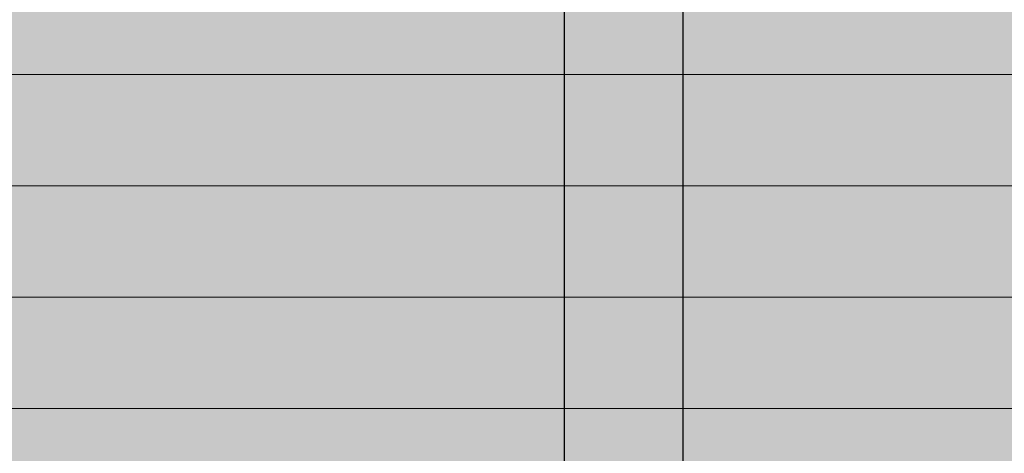
# Model space of a CAD drawing. Units: inches. Extents: x 1704 to 6393, y -157 to 1172.
# Tile 98 of 122: x 2561 to 2627, y 972 to 1001. Entities that reach past the tile are written whole.
import ezdxf

# ---------------------------------------------------------------- set-up
doc = ezdxf.new("R2010")
doc.units = ezdxf.units.IN
doc.header["$MEASUREMENT"] = 0
doc.layers.add('A-ANNO-DIMS', color=7, linetype='Continuous', lineweight=13)
doc.layers.add('L-DECK-PLNK-PATT', color=250, linetype='Continuous', lineweight=13)
doc.layers.add('L-DECK-PATT', color=35, linetype='Continuous', lineweight=13, true_color=0xa6725b)
doc.styles.get("Standard").update_dxf_attribs({"font": 'arial.ttf'})
doc.dimstyles.get("Standard").update_dxf_attribs({"dimtxt": 6, "dimasz": 2, "dimexe": 0.18, "dimexo": 0.0625, "dimgap": 0.09, "dimtad": 0, "dimtih": 1, "dimtoh": 1, "dimdec": 1, "dimzin": 0, "dimdsep": 46, "dimlunit": 3, "dimtxsty": 'Standard', "dimblk": 'ARCHTICK', "dimcen": 0.09, "dimadec": 0, "dimazin": 0, "dimtfac": 1, "dimtdec": 1, "dimtofl": 0, "dimtmove": 0, "dimatfit": 3, "dimfxl": 1, "dimtolj": 1, "dimtzin": 0, "dimarcsym": 0})

# ---------------------------------------------------------------- blocks, each defined once
blk = doc.blocks.new('_ArchTick')
at = {"color": 0, "linetype": 'ByBlock', "const_width": 0.15}
blk.add_lwpolyline([(-0.5, -0.5), (0.5, 0.5)], dxfattribs=at)
blk = doc.blocks.new('*D92')
at = {"layer": 'A-ANNO-DIMS', "color": 0, "lineweight": -2, "transparency": 16777216}
for p, q in [((2073.349, 895.275), (2073.349, 1105.287)), ((2605.349, 895.275), (2605.349, 1105.287)), ((2073.349, 1105.107), (2332.661, 1105.107)), ((2605.349, 1105.107), (2346.036, 1105.107))]:
    blk.add_line(p, q, dxfattribs=at)
at = {"layer": 'Defpoints', "color": 0, "lineweight": -3, "transparency": 16777216}
for p in [(2605.349, 1105.107), (2073.349, 895.213), (2605.349, 895.213)]:
    blk.add_point(p, dxfattribs=at)
at = {"layer": 'A-ANNO-DIMS', "color": 0, "lineweight": -2, "transparency": 16777216, "xscale": 2, "yscale": 2, "zscale": 2, "rotation": 180}
blk.add_blockref('_ArchTick', (2073.349, 1105.107), dxfattribs=at)
at = {"layer": 'A-ANNO-DIMS', "color": 0, "lineweight": -2, "transparency": 16777216, "xscale": 2, "yscale": 2, "zscale": 2}
blk.add_blockref('_ArchTick', (2605.349, 1105.107), dxfattribs=at)
at = {"layer": 'A-ANNO-DIMS', "color": 0, "transparency": 16777216, "insert": (2339.349, 1105.107), "char_height": 6, "attachment_point": 5}
blk.add_mtext('\\A1;532', dxfattribs=at)
blk = doc.blocks.new('*D95')
at = {"layer": 'A-ANNO-DIMS', "color": 0, "lineweight": -2, "transparency": 16777216}
for p, q in [((2605.349, 895.275), (2605.349, 1105.287)), ((2723.349, 895.275), (2723.349, 1105.287)), ((2605.349, 1105.107), (2657.907, 1105.107)), ((2723.349, 1105.107), (2670.791, 1105.107))]:
    blk.add_line(p, q, dxfattribs=at)
at = {"layer": 'Defpoints', "color": 0, "lineweight": -3, "transparency": 16777216}
for p in [(2723.349, 1105.107), (2605.349, 895.213), (2723.349, 895.213)]:
    blk.add_point(p, dxfattribs=at)
at = {"layer": 'A-ANNO-DIMS', "color": 0, "lineweight": -2, "transparency": 16777216, "xscale": 2, "yscale": 2, "zscale": 2, "rotation": 180}
blk.add_blockref('_ArchTick', (2605.349, 1105.107), dxfattribs=at)
at = {"layer": 'A-ANNO-DIMS', "color": 0, "lineweight": -2, "transparency": 16777216, "xscale": 2, "yscale": 2, "zscale": 2}
blk.add_blockref('_ArchTick', (2723.349, 1105.107), dxfattribs=at)
at = {"layer": 'A-ANNO-DIMS', "color": 0, "transparency": 16777216, "insert": (2664.349, 1105.107), "char_height": 6, "attachment_point": 5}
blk.add_mtext('\\A1;118', dxfattribs=at)
blk = doc.blocks.new('*D103')
at = {"layer": 'A-ANNO-DIMS', "color": 0, "lineweight": -2, "transparency": 16777216}
for p, q in [((2551.349, 711.275), (2551.349, 1105.287)), ((2597.349, 711.275), (2597.349, 1105.287)), ((2551.349, 1105.107), (2569.842, 1105.107)), ((2597.349, 1105.107), (2578.855, 1105.107))]:
    blk.add_line(p, q, dxfattribs=at)
at = {"layer": 'Defpoints', "color": 0, "lineweight": -3, "transparency": 16777216}
for p in [(2597.349, 1105.107), (2551.349, 711.213), (2597.349, 711.213)]:
    blk.add_point(p, dxfattribs=at)
at = {"layer": 'A-ANNO-DIMS', "color": 0, "lineweight": -2, "transparency": 16777216, "xscale": 2, "yscale": 2, "zscale": 2, "rotation": 180}
blk.add_blockref('_ArchTick', (2551.349, 1105.107), dxfattribs=at)
at = {"layer": 'A-ANNO-DIMS', "color": 0, "lineweight": -2, "transparency": 16777216, "xscale": 2, "yscale": 2, "zscale": 2}
blk.add_blockref('_ArchTick', (2597.349, 1105.107), dxfattribs=at)
at = {"layer": 'A-ANNO-DIMS', "color": 0, "transparency": 16777216, "insert": (2574.349, 1105.107), "char_height": 6, "attachment_point": 5}
blk.add_mtext('\\A1;46', dxfattribs=at)

msp = doc.modelspace()

# ---------------------------------------------------------------- hatches: boundary and pattern name
at = {"layer": 'L-DECK-PATT', "transparency": 33554544}
h = msp.add_hatch(color=256, dxfattribs=at)
h.dxf.hatch_style = 1
h.paths.add_polyline_path([(2329.589, 1033.213), (2065.589, 1033.213), (2065.589, 895.213), (2167.349, 895.213), (2263.349, 895.213), (2263.349, 903.213), (2273.349, 903.213), (2273.349, 895.213), (2329.589, 895.213)])
h.paths.add_polyline_path([(2664.349, 1033.213), (2333.589, 1033.213), (2333.589, 895.213), (2465.349, 895.213), (2469.181, 895.213), (2470.482, 895.213), (2508.215, 895.213), (2509.516, 895.213), (2513.349, 895.213), (2533.349, 895.213), (2581.349, 895.213), (2605.349, 895.213), (2664.349, 895.213)])
h.paths.add_polyline_path([(2333.589, 1033.213), (2329.589, 1033.213), (2329.589, 895.213), (2333.589, 895.213)])
at = {"layer": 'L-DECK-PLNK-PATT'}
h = msp.add_hatch(dxfattribs=at)
h.set_pattern_fill('LINE', color=256, scale=60)
h.paths.add_polyline_path([(2329.589, 1033.213), (2065.589, 1033.213), (2065.589, 895.213), (2167.349, 895.213), (2263.349, 895.213), (2263.349, 903.213), (2273.349, 903.213), (2273.349, 895.213), (2329.589, 895.213)])
h.paths.add_polyline_path([(2664.349, 1033.213), (2333.589, 1033.213), (2333.589, 895.213), (2465.349, 895.213), (2469.181, 895.213), (2470.482, 895.213), (2508.215, 895.213), (2509.516, 895.213), (2513.349, 895.213), (2533.349, 895.213), (2581.349, 895.213), (2605.349, 895.213), (2664.349, 895.213)])
h.paths.add_polyline_path([(2333.589, 1033.213), (2329.589, 1033.213), (2329.589, 895.213), (2333.589, 895.213)])

# ---------------------------------------------------------------- dimensions: what is measured, and where the dimension line sits
at = {"layer": 'A-ANNO-DIMS'}
for base, p1, p2, picture, middle in [((2605.349, 1105.107), (2073.349, 895.213), (2605.349, 895.213), '*D92', (2339.349, 1105.107)), ((2597.349, 1105.107), (2551.349, 711.213), (2597.349, 711.213), '*D103', (2574.349, 1105.107)), ((2723.349, 1105.107), (2605.349, 895.213), (2723.349, 895.213), '*D95', (2664.349, 1105.107))]:
    dim = msp.add_linear_dim(base=base, p1=p1, p2=p2, dimstyle='Standard', override={"dimdec": 0, "dimlfac": 1, "dimrnd": 0, "dimzin": 0, "dimdsep": 46, "dimlunit": 2}, dxfattribs=at)
    dim.commit()
    dim.dimension.update_dxf_attribs({"geometry": picture, "text_midpoint": middle})

doc.saveas('drawing.dxf')
